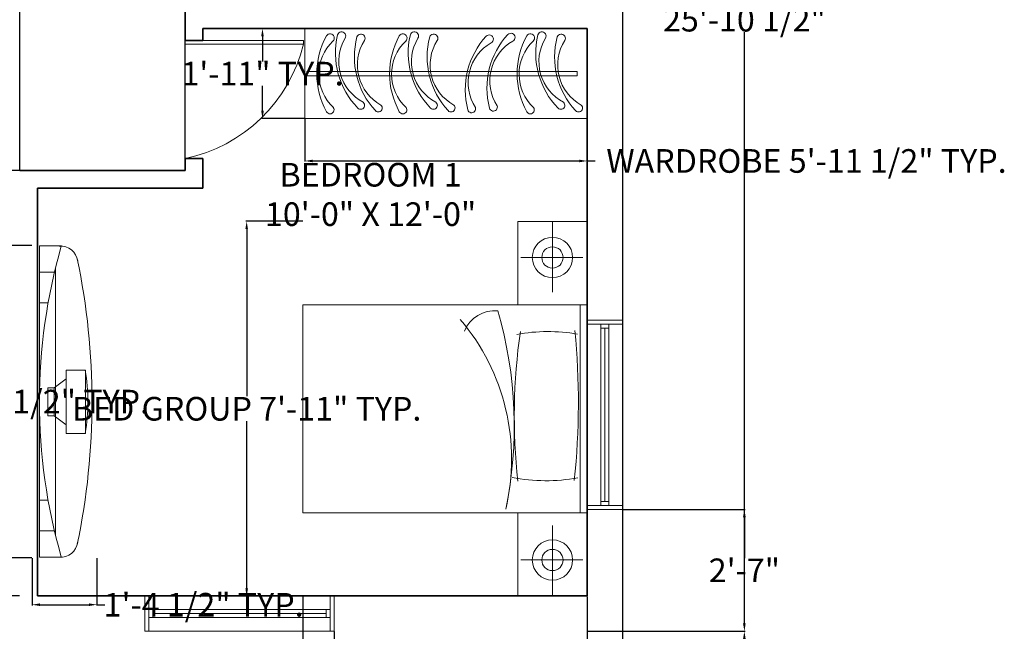
# Model space of a CAD drawing. Units: inches. Extents: x 84 to 590, y 32 to 648.
# Tile 4 of 6: x 340 to 590, y 245 to 401. Entities that reach past the tile are written whole.
import ezdxf

# ---------------------------------------------------------------- set-up
doc = ezdxf.new("R2010")
doc.units = ezdxf.units.IN
doc.header["$MEASUREMENT"] = 0
for name, color, linetype, lineweight in [('A-ANNO-DIMS', 2, 'Continuous', 18), ('A-AREA-IDEN', 7, 'Continuous', 18), ('A-DOOR', 4, 'Continuous', 18), ('A-FLOR-CASE', 9, 'Continuous', 18), ('A-FURN', 8, 'Continuous', 18), ('A-GLAZ', 4, 'Continuous', 18), ('A-WALL', 7, 'Continuous', 35), ('C-PROP', 7, 'Continuous', 30)]:
    doc.layers.add(name, color=color, linetype=linetype, lineweight=lineweight)
doc.styles.get("Standard").update_dxf_attribs({"font": 'arial.ttf'})
doc.dimstyles.get("Standard").update_dxf_attribs({"dimtxt": 6, "dimasz": 2, "dimexe": 0.18, "dimexo": 0.0625, "dimgap": 0.09, "dimtad": 0, "dimtih": 1, "dimtoh": 1, "dimdec": 0, "dimzin": 0, "dimdsep": 46, "dimlunit": 4, "dimtxsty": 'Standard', "dimcen": 0.09, "dimadec": 0, "dimazin": 0, "dimtfac": 1, "dimtdec": 0, "dimtofl": 0, "dimtmove": 0, "dimatfit": 3, "dimfxl": 1, "dimtolj": 1, "dimtzin": 0, "dimarcsym": 1})

# ---------------------------------------------------------------- blocks, each defined once
blk = doc.blocks.new('DOOR')
for p, q in [((185.51, 1128.53), (185.51, 1098.53)), ((185.51, 1128.53), (186.51, 1128.53)), ((186.51, 1098.53), (186.51, 1128.53)), ((186.51, 1098.53), (156.51, 1098.53))]:
    blk.add_line(p, q)
blk.add_arc((194.73, 1090.6), 39.03, 103.6607, 168.2814)
blk = doc.blocks.new('CVBNM')
for p, q in [((388.24, 1592.71), (388.24, 1565.71)), ((420.64, 1592.71), (388.24, 1592.71)), ((420.64, 1592.71), (420.64, 1568.41)), ((420.64, 1482.01), (420.64, 1592.71)), ((501.64, 1592.71), (420.64, 1592.71)), ((420.64, 1565.71), (420.64, 1592.71)), ((501.64, 1592.71), (501.64, 1568.41)), ((501.64, 1592.71), (501.64, 1568.41)), ((501.64, 1482.01), (501.64, 1592.71)), ((501.64, 1565.71), (501.64, 1592.71)), ((501.64, 1592.71), (534.04, 1592.71)), ((534.04, 1592.71), (534.04, 1565.71)), ((402.21, 1579.21), (402.21, 1591.06)), ((501.64, 1590.01), (420.64, 1590.01)), ((520.07, 1579.21), (520.07, 1591.06)), ((402.21, 1579.21), (388.08, 1579.21)), ((402.21, 1579.21), (415.71, 1579.21)), ((402.21, 1579.21), (402.21, 1566.9)), ((520.07, 1579.21), (506.57, 1579.21)), ((520.07, 1579.21), (534.21, 1579.21)), ((520.07, 1579.21), (520.07, 1566.9)), ((388.24, 1565.71), (420.64, 1565.71)), ((534.04, 1565.71), (501.64, 1565.71)), ((501.64, 1482.01), (420.64, 1482.01))]:
    blk.add_line(p, q)
for centre, radius in [((402.21, 1579.21), 7.85), ((520.07, 1579.21), 7.85), ((402.21, 1579.21), 4.15), ((520.07, 1579.21), 4.15)]:
    blk.add_circle(centre, radius)
for centre, radius, start, end in [((458.61, 1300.37), 288.94, 83.953, 95.5626), ((496.51, 1577.48), 65.44, 169.9145, 190.6851), ((419.34, 1576.61), 69.84, 349.1761, 10.2706), ((464.08, 1794.56), 230.23, 261.7649, 276.2896), ((467.83, 1404.8), 159.53, 78.2462, 106.3473), ((480.78, 1479.19), 84.09, 76.5636, 130.3236), ((435.77, 1556.83), 12.88, 175.3269, 247.5588)]:
    blk.add_arc(centre, radius, start, end)
blk = doc.blocks.new('A$C20D7642B')
for p, q in [((0, 1879.7), (0, 0)), ((600, 1879.7), (0, 1879.7)), ((600, 1879.7), (600, 0)), ((285.2, 14), (285.2, 1812.3)), ((285.2, 1812.3), (316, 1812.3)), ((316, 1812.3), (316, 14)), ((340, 0), (0, 0)), ((316, 14), (285.2, 14)), ((340, 0), (600, 0))]:
    blk.add_line(p, q)
for centre, radius, start, end in [((242.6, 1988.3), 305.1, 237.78554, 330.91711), ((529.2, 1822.6), 26.4, 312.06888, 138.87685), ((189.7, 2189.4), 526.2, 255.30638, 312.74923), ((64.5, 1707), 27.8, 56.33784, 252.73759), ((220.7, 1863.8), 305.1, 239.17077, 332.30233), ((511.2, 1705.1), 26.4, 313.4541, 140.26207), ((163, 2063.5), 526.2, 256.69161, 314.13445), ((49.5, 1578.3), 27.8, 57.72306, 254.12281), ((62.8, 1501.9), 27.8, 42.31003, 238.70978), ((303.8, 1731.6), 305.1, 223.75774, 316.8893), ((541.6, 1501.4), 26.4, 298.04107, 124.84904), ((301.2, 1939.5), 526.2, 241.27858, 298.72142), ((59.1, 1372.1), 27.8, 28.28014, 224.67989), ((348.6, 1536.6), 305.1, 209.72784, 302.85941), ((396.5, 1738.9), 526.2, 227.24868, 284.69153), ((70.6, 1227.4), 27.8, 28.28014, 224.67989), ((523.6, 1255.6), 26.4, 284.01118, 110.81915), ((408, 1594.2), 526.2, 227.24868, 284.69153), ((360, 1391.9), 305.1, 209.72784, 302.85941), ((535, 1110.9), 26.4, 284.01118, 110.81915), ((242.6, 1139.3), 305.1, 237.78554, 330.91711), ((529.2, 973.6), 26.4, 312.06888, 138.87685), ((189.7, 1340.3), 526.2, 255.30638, 312.74923), ((64.5, 857.9), 27.8, 56.33784, 252.73759), ((220.7, 1014.8), 305.1, 239.17077, 332.30233), ((511.2, 856), 26.4, 313.4541, 140.26207), ((163, 1214.5), 526.2, 256.69161, 314.13445), ((49.5, 729.2), 27.8, 57.72306, 254.12281), ((62.8, 652.8), 27.8, 42.31003, 238.70978), ((303.8, 882.6), 305.1, 223.75774, 316.8893), ((541.6, 652.4), 26.4, 298.04107, 124.84904), ((301.2, 1090.5), 526.2, 241.27858, 298.72142), ((189.7, 856), 526.2, 255.30638, 312.74923), ((242.6, 655), 305.1, 237.78554, 330.91711), ((529.2, 489.2), 26.4, 312.06888, 138.87685), ((64.5, 373.6), 27.8, 56.33784, 252.73759), ((511.2, 371.7), 26.4, 313.4541, 140.26207), ((163, 730.2), 526.2, 256.69161, 314.13445), ((220.7, 530.5), 305.1, 239.17077, 332.30233), ((49.5, 244.9), 27.8, 57.72306, 254.12281), ((62.8, 168.5), 27.8, 42.31003, 238.70978), ((301.2, 606.1), 526.2, 241.27858, 298.72142), ((303.8, 398.3), 305.1, 223.75774, 316.8893), ((541.6, 168), 26.4, 298.04107, 124.84904)]:
    blk.add_arc(centre, radius, start, end)
blk = doc.blocks.new('A$C78AE5658')
for p, q in [((1515, 306), (1515, 524)), ((1515, 524), (2236, 524)), ((2236, 306), (2236, 524)), ((98, 250), (98, 252)), ((98, 250), (98, 0)), ((1515, 306), (2236, 306)), ((1613, 306), (1716, 168)), ((2137, 306), (2034, 168)), ((3648, 250), (3648, 252)), ((3648, 0), (3648, 250)), ((348, 184), (3398, 184)), ((398, 0), (398, 172)), ((2034, 168), (1716, 168)), ((1716, 168), (1716, 98)), ((2034, 168), (2034, 98)), ((3348, 0), (3348, 172)), ((3648, 0), (98, 0)), ((748, 0), (748, 99)), ((2034, 98), (1716, 98)), ((2998, 0), (2998, 99))]:
    blk.add_line(p, q)
blk.add_lwpolyline([(246, 432, -0.103184), (3500, 432, -0.103184)], format="xyb")
for centre, radius, start, end in [((1875, -1675), 2228, 80.6925, 99.3075), ((298, 239), 200, 98.4687, 183.693), ((3449, 239), 200, 356.307, 81.5313), ((1873, 6426), 6426, 253.9658, 286.0342)]:
    blk.add_arc(centre, radius, start, end)
blk = doc.blocks.new('WIND')
for p, q in [((-51.89, 1021.98), (-99.89, 1021.98)), ((-99.89, 1021.98), (-99.89, 1012.98)), ((-98.89, 1021.98), (-98.89, 1012.98)), ((-52.89, 1012.98), (-52.89, 1021.98)), ((-51.89, 1012.98), (-51.89, 1021.98)), ((-98.89, 1018.48), (-52.89, 1018.48)), ((-97.89, 1018.48), (-97.89, 1016.48)), ((-97.89, 1017.48), (-53.89, 1017.48)), ((-53.89, 1016.48), (-53.89, 1018.48)), ((-98.89, 1016.48), (-52.89, 1016.48)), ((-99.89, 1012.98), (-51.89, 1012.98))]:
    blk.add_line(p, q)
blk = doc.blocks.new('*D23')
at = {"layer": 'A-ANNO-DIMS', "color": 0, "lineweight": -2, "transparency": 16777216}
for p, q in [((411.85, 349.43), (397.45, 349.43)), ((397.63, 347.43), (397.63, 305.03)), ((397.63, 256.23), (397.63, 298.64)), ((411.85, 254.23), (397.45, 254.23))]:
    blk.add_line(p, q, dxfattribs=at)
at = {"layer": 'A-ANNO-DIMS', "color": 0, "transparency": 16777216}
for points in [[(397.3, 347.43), (397.96, 347.43), (397.63, 349.43)], [(397.3, 256.23), (397.96, 256.23), (397.63, 254.23)]]:
    blk.add_solid(points, dxfattribs=at)
at = {"layer": 'Defpoints', "color": 0, "transparency": 16777216}
for p in [(411.91, 349.43), (397.63, 254.23), (411.91, 254.23)]:
    blk.add_point(p, dxfattribs=at)
at = {"layer": 'A-ANNO-DIMS', "color": 0, "transparency": 16777216, "insert": (397.63, 301.83), "char_height": 6, "attachment_point": 5}
blk.add_mtext('\\A1;BED GROUP 7\'-11" TYP.', dxfattribs=at)
blk = doc.blocks.new('*D24')
at = {"layer": 'A-ANNO-DIMS', "color": 0, "lineweight": -2, "transparency": 16777216}
for p, q in [((411.91, 254.17), (411.91, 239.77)), ((484.03, 254.17), (484.03, 239.77)), ((413.91, 239.95), (429.58, 239.95)), ((482.03, 239.95), (466.36, 239.95))]:
    blk.add_line(p, q, dxfattribs=at)
at = {"layer": 'A-ANNO-DIMS', "color": 0, "transparency": 16777216}
for points in [[(413.91, 240.28), (413.91, 239.62), (411.91, 239.95)], [(482.03, 240.28), (482.03, 239.62), (484.03, 239.95)]]:
    blk.add_solid(points, dxfattribs=at)
at = {"layer": 'Defpoints', "color": 0, "transparency": 16777216}
for p in [(411.91, 254.23), (484.03, 254.23), (484.03, 239.95)]:
    blk.add_point(p, dxfattribs=at)
at = {"layer": 'A-ANNO-DIMS', "color": 0, "transparency": 16777216, "insert": (447.97, 239.95), "char_height": 6, "attachment_point": 5}
blk.add_mtext('\\A1;6\'-0" TYP.', dxfattribs=at)
blk = doc.blocks.new('*D25')
at = {"layer": 'A-ANNO-DIMS', "color": 0, "lineweight": -2, "transparency": 16777216}
for p, q in [((343.11, 343.29), (331.1, 343.29)), ((331.28, 341.29), (331.28, 306.83)), ((331.28, 265.98), (331.28, 300.44)), ((343.11, 263.98), (331.1, 263.98))]:
    blk.add_line(p, q, dxfattribs=at)
at = {"layer": 'A-ANNO-DIMS', "color": 0, "transparency": 16777216}
for points in [[(330.95, 341.29), (331.61, 341.29), (331.28, 343.29)], [(330.95, 265.98), (331.61, 265.98), (331.28, 263.98)]]:
    blk.add_solid(points, dxfattribs=at)
at = {"layer": 'Defpoints', "color": 0, "transparency": 16777216}
for p in [(343.17, 343.29), (331.28, 263.98), (343.17, 263.98)]:
    blk.add_point(p, dxfattribs=at)
at = {"layer": 'A-ANNO-DIMS', "color": 0, "transparency": 16777216, "insert": (331.28, 303.64), "char_height": 6, "attachment_point": 5}
blk.add_mtext('\\A1;TV UNIT 6\'-7 1/2" TYP.', dxfattribs=at)
blk = doc.blocks.new('*D26')
at = {"layer": 'A-ANNO-DIMS', "color": 0, "lineweight": -2, "transparency": 16777216}
for p, q in [((343.17, 263.92), (343.17, 251.91)), ((359.62, 263.92), (359.62, 251.91)), ((345.17, 252.09), (357.62, 252.09)), ((359.62, 252.09), (361.62, 252.09))]:
    blk.add_line(p, q, dxfattribs=at)
at = {"layer": 'A-ANNO-DIMS', "color": 0, "transparency": 16777216}
for points in [[(345.17, 252.42), (345.17, 251.76), (343.17, 252.09)], [(357.62, 252.42), (357.62, 251.76), (359.62, 252.09)]]:
    blk.add_solid(points, dxfattribs=at)
at = {"layer": 'Defpoints', "color": 0, "transparency": 16777216}
for p in [(343.17, 263.98), (359.62, 263.98), (359.62, 252.09)]:
    blk.add_point(p, dxfattribs=at)
at = {"layer": 'A-ANNO-DIMS', "color": 0, "transparency": 16777216, "insert": (386.71, 252.09), "char_height": 6, "attachment_point": 5}
blk.add_mtext('\\A1;1\'-4 1/2" TYP.', dxfattribs=at)
blk = doc.blocks.new('*D27')
at = {"layer": 'A-ANNO-DIMS', "color": 0, "lineweight": -2, "transparency": 16777216}
for p, q in [((412.39, 375.41), (412.39, 364.55)), ((484.03, 375.41), (484.03, 364.55)), ((414.39, 364.73), (482.03, 364.73)), ((484.03, 364.73), (486.03, 364.73))]:
    blk.add_line(p, q, dxfattribs=at)
at = {"layer": 'A-ANNO-DIMS', "color": 0, "transparency": 16777216}
for points in [[(414.39, 365.06), (414.39, 364.39), (412.39, 364.73)], [(482.03, 365.06), (482.03, 364.39), (484.03, 364.73)]]:
    blk.add_solid(points, dxfattribs=at)
at = {"layer": 'Defpoints', "color": 0, "transparency": 16777216}
for p in [(412.39, 375.47), (484.03, 375.47), (484.03, 364.73)]:
    blk.add_point(p, dxfattribs=at)
at = {"layer": 'A-ANNO-DIMS', "color": 0, "transparency": 16777216, "insert": (539.69, 364.73), "char_height": 6, "attachment_point": 5}
blk.add_mtext('\\A1;WARDROBE 5\'-11 1/2" TYP.', dxfattribs=at)
blk = doc.blocks.new('*D28')
at = {"layer": 'A-ANNO-DIMS', "color": 0, "lineweight": -2, "transparency": 16777216}
for p, q in [((412.33, 398.34), (401.46, 398.34)), ((401.64, 396.34), (401.64, 390.01)), ((401.64, 377.47), (401.64, 383.8)), ((412.33, 375.47), (401.46, 375.47))]:
    blk.add_line(p, q, dxfattribs=at)
at = {"layer": 'A-ANNO-DIMS', "color": 0, "transparency": 16777216}
for points in [[(401.31, 396.34), (401.98, 396.34), (401.64, 398.34)], [(401.31, 377.47), (401.98, 377.47), (401.64, 375.47)]]:
    blk.add_solid(points, dxfattribs=at)
at = {"layer": 'Defpoints', "color": 0, "transparency": 16777216}
for p in [(412.39, 398.34), (401.64, 375.47), (412.39, 375.47)]:
    blk.add_point(p, dxfattribs=at)
at = {"layer": 'A-ANNO-DIMS', "color": 0, "transparency": 16777216, "insert": (401.64, 386.9), "char_height": 6, "attachment_point": 5}
blk.add_mtext('\\A1;1\'-11" TYP.', dxfattribs=at)
blk = doc.blocks.new('*D44')
at = {"layer": 'A-ANNO-DIMS', "color": 0, "lineweight": -2, "transparency": 16777216}
for p, q in [((484.09, 555.84), (524.11, 555.84)), ((523.93, 553.84), (523.93, 403.78)), ((523.93, 247.34), (523.93, 397.4)), ((484.09, 245.34), (524.11, 245.34))]:
    blk.add_line(p, q, dxfattribs=at)
at = {"layer": 'A-ANNO-DIMS', "color": 0, "transparency": 16777216}
for points in [[(523.59, 553.84), (524.26, 553.84), (523.93, 555.84)], [(523.59, 247.34), (524.26, 247.34), (523.93, 245.34)]]:
    blk.add_solid(points, dxfattribs=at)
at = {"layer": 'Defpoints', "color": 0, "transparency": 16777216}
for p in [(484.03, 555.84), (484.03, 245.34), (523.93, 245.34)]:
    blk.add_point(p, dxfattribs=at)
at = {"layer": 'A-ANNO-DIMS', "color": 0, "transparency": 16777216, "insert": (523.93, 400.59), "char_height": 6, "attachment_point": 5}
blk.add_mtext('\\A1;25\'-10 1/2"', dxfattribs=at)
blk = doc.blocks.new('*D45')
at = {"layer": 'A-ANNO-DIMS', "color": 0, "lineweight": -2, "transparency": 16777216}
for p, q in [((484.09, 245.34), (524.11, 245.34)), ((523.93, 243.34), (523.93, 177.99)), ((523.93, 106.34), (523.93, 171.68)), ((493.09, 104.34), (524.11, 104.34))]:
    blk.add_line(p, q, dxfattribs=at)
at = {"layer": 'A-ANNO-DIMS', "color": 0, "transparency": 16777216}
for points in [[(523.59, 243.34), (524.26, 243.34), (523.93, 245.34)], [(523.59, 106.34), (524.26, 106.34), (523.93, 104.34)]]:
    blk.add_solid(points, dxfattribs=at)
at = {"layer": 'Defpoints', "color": 0, "transparency": 16777216}
for p in [(484.03, 245.34), (493.03, 104.34), (523.93, 104.34)]:
    blk.add_point(p, dxfattribs=at)
at = {"layer": 'A-ANNO-DIMS', "color": 0, "transparency": 16777216, "insert": (523.93, 174.84), "char_height": 6, "attachment_point": 5}
blk.add_mtext('\\A1;11\'-9"', dxfattribs=at)
blk = doc.blocks.new('*D55')
at = {"layer": 'A-ANNO-DIMS', "color": 0, "lineweight": -2, "transparency": 16777216}
for p, q in [((493.09, 276.3), (524.11, 276.3)), ((523.93, 274.3), (523.93, 263.92)), ((523.93, 247.34), (523.93, 257.72)), ((484.09, 245.34), (524.11, 245.34))]:
    blk.add_line(p, q, dxfattribs=at)
at = {"layer": 'A-ANNO-DIMS', "color": 0, "transparency": 16777216}
for points in [[(523.59, 274.3), (524.26, 274.3), (523.93, 276.3)], [(523.59, 247.34), (524.26, 247.34), (523.93, 245.34)]]:
    blk.add_solid(points, dxfattribs=at)
at = {"layer": 'Defpoints', "color": 0, "transparency": 16777216}
for p in [(493.03, 276.3), (523.93, 276.3), (484.03, 245.34)]:
    blk.add_point(p, dxfattribs=at)
at = {"layer": 'A-ANNO-DIMS', "color": 0, "transparency": 16777216, "insert": (523.93, 260.82), "char_height": 6, "attachment_point": 5}
blk.add_mtext('\\A1;2\'-7"', dxfattribs=at)
blk = doc.blocks.new('*D59')
at = {"layer": 'A-ANNO-DIMS', "color": 0, "lineweight": -2, "transparency": 16777216}
for p, q in [((419.82, 245.28), (419.82, 73.26)), ((484.03, 245.28), (484.03, 73.26)), ((421.82, 73.44), (443.86, 73.44)), ((482.03, 73.44), (459.99, 73.44))]:
    blk.add_line(p, q, dxfattribs=at)
at = {"layer": 'A-ANNO-DIMS', "color": 0, "transparency": 16777216}
for points in [[(421.82, 73.77), (421.82, 73.1), (419.82, 73.44)], [(482.03, 73.77), (482.03, 73.1), (484.03, 73.44)]]:
    blk.add_solid(points, dxfattribs=at)
at = {"layer": 'Defpoints', "color": 0, "transparency": 16777216}
for p in [(419.82, 245.34), (484.03, 245.34), (484.03, 73.44)]:
    blk.add_point(p, dxfattribs=at)
at = {"layer": 'A-ANNO-DIMS', "color": 0, "transparency": 16777216, "insert": (451.92, 73.44), "char_height": 6, "attachment_point": 5}
blk.add_mtext('\\A1;5\'-4"', dxfattribs=at)
blk = doc.blocks.new('*D60')
at = {"layer": 'A-ANNO-DIMS', "color": 0, "lineweight": -2, "transparency": 16777216}
for p, q in [((340.03, 362.4), (340.03, 639.42)), ((342.03, 639.24), (352.97, 639.24)), ((380.03, 639.24), (369.09, 639.24)), ((382.03, 362.4), (382.03, 639.42))]:
    blk.add_line(p, q, dxfattribs=at)
at = {"layer": 'A-ANNO-DIMS', "color": 0, "transparency": 16777216}
for points in [[(342.03, 639.57), (342.03, 638.9), (340.03, 639.24)], [(380.03, 639.57), (380.03, 638.9), (382.03, 639.24)]]:
    blk.add_solid(points, dxfattribs=at)
at = {"layer": 'Defpoints', "color": 0, "transparency": 16777216}
for p in [(382.03, 639.24), (340.03, 362.34), (382.03, 362.34)]:
    blk.add_point(p, dxfattribs=at)
at = {"layer": 'A-ANNO-DIMS', "color": 0, "transparency": 16777216, "insert": (361.03, 639.24), "char_height": 6, "attachment_point": 5}
blk.add_mtext('\\A1;3\'-6"', dxfattribs=at)
blk = doc.blocks.new('*D61')
at = {"layer": 'A-ANNO-DIMS', "color": 0, "lineweight": -2, "transparency": 16777216}
for p, q in [((339.97, 362.34), (101.95, 362.34)), ((102.13, 360.34), (102.13, 311.49)), ((102.13, 256.34), (102.13, 305.18)), ((339.97, 254.34), (101.95, 254.34))]:
    blk.add_line(p, q, dxfattribs=at)
at = {"layer": 'A-ANNO-DIMS', "color": 0, "transparency": 16777216}
for points in [[(101.79, 360.34), (102.46, 360.34), (102.13, 362.34)], [(101.79, 256.34), (102.46, 256.34), (102.13, 254.34)]]:
    blk.add_solid(points, dxfattribs=at)
at = {"layer": 'Defpoints', "color": 0, "transparency": 16777216}
for p in [(102.13, 362.34), (340.03, 362.34), (340.03, 254.34)]:
    blk.add_point(p, dxfattribs=at)
at = {"layer": 'A-ANNO-DIMS', "color": 0, "transparency": 16777216, "insert": (102.13, 308.34), "char_height": 6, "attachment_point": 5}
blk.add_mtext('\\A1;9\'-0"', dxfattribs=at)

msp = doc.modelspace()

# ---------------------------------------------------------------- linework, layer by layer
at = {"layer": 'A-WALL'}
for p, q in [((382.03, 398.34), (382.03, 408.84)), ((382.03, 398.34), (382.03, 395.34)), ((386.53, 398.34), (484.03, 398.34)), ((386.53, 398.34), (386.53, 395.34)), ((484.03, 398.34), (484.03, 254.34)), ((382.03, 395.34), (386.53, 395.34)), ((382.03, 365.34), (386.53, 365.34)), ((382.03, 365.34), (382.03, 362.34)), ((386.53, 365.34), (386.53, 357.84)), ((382.03, 362.34), (340.03, 362.34)), ((344.53, 254.34), (344.53, 357.84)), ((386.53, 357.84), (344.53, 357.84)), ((344.53, 254.34), (484.03, 254.34))]:
    msp.add_line(p, q, dxfattribs=at)
at = {"layer": 'C-PROP'}
msp.add_line((493.03, 608.34), (493.03, 104.34), dxfattribs=at)

# ---------------------------------------------------------------- block references
at = {"layer": 'A-DOOR', "xscale": -1, "rotation": 270}
msp.add_blockref('DOOR', (-716.5, 208.83), dxfattribs=at)
at = {"layer": 'A-FLOR-CASE', "xscale": 0.0381118678123285, "yscale": 0.0381118678123285, "zscale": 0.0381118678123285, "rotation": 270}
msp.add_blockref('A$C20D7642B', (412.39, 398.34), dxfattribs=at)
at = {"layer": 'A-FURN', "rotation": 270}
for name, p, xscale, yscale, zscale in [('CVBNM', (-553.6, 602.26), 0.6514848881435277, 0.6514848881435277, 0.6514848881435277), ('A$C78AE5658', (345.03, 345.33), 0.0222542726180731, 0.0222542726180731, 0.0222542726180731)]:
    msp.add_blockref(name, p, dxfattribs=dict(at, xscale=xscale, yscale=yscale, zscale=zscale))
at = {"layer": 'A-GLAZ', "rotation": 270}
msp.add_blockref('WIND', (-528.95, 224.4), dxfattribs=at)
at = {"layer": 'A-GLAZ'}
msp.add_blockref('WIND', (471.71, -767.64), dxfattribs=at)

# ---------------------------------------------------------------- texts
at = {"layer": 'A-AREA-IDEN', "insert": (387.96, 364.23), "char_height": 6, "attachment_point": 1}
msp.add_mtext_dynamic_manual_height_columns('\\pxqc;BEDROOM 1\\P10\'-0" X 12\'-0"', width=82.2238, gutter_width=30, heights=[0], dxfattribs=at)

# ---------------------------------------------------------------- dimensions: what is measured, and where the dimension line sits
at = {"layer": 'A-ANNO-DIMS'}
for base, p1, p2, picture, middle in [((382.03, 639.24), (340.03, 362.34), (382.03, 362.34), '*D60', (361.03, 639.24)), ((484.03, 73.44), (419.82, 245.34), (484.03, 245.34), '*D59', (451.92, 73.44))]:
    dim = msp.add_linear_dim(base=base, p1=p1, p2=p2, dimstyle='Standard', override={"dimdec": 1, "dimlfac": 1, "dimrnd": 0, "dimzin": 1, "dimdsep": 46, "dimlunit": 4, "dimfrac": 2}, dxfattribs=at)
    dim.commit()
    dim.dimension.update_dxf_attribs({"geometry": picture, "text_midpoint": middle})
for base, p1, p2, picture, middle in [((523.93, 245.34), (484.03, 555.84), (484.03, 245.34), '*D44', (523.93, 400.59)), ((102.13, 362.34), (340.03, 254.34), (340.03, 362.34), '*D61', (102.13, 308.34)), ((523.93, 276.3), (484.03, 245.34), (493.03, 276.3), '*D55', (523.93, 260.82)), ((523.93, 104.34), (484.03, 245.34), (493.03, 104.34), '*D45', (523.93, 174.84))]:
    dim = msp.add_linear_dim(base=base, p1=p1, p2=p2, angle=90, dimstyle='Standard', override={"dimdec": 1, "dimlfac": 1, "dimrnd": 0, "dimzin": 1, "dimdsep": 46, "dimlunit": 4, "dimfrac": 2}, dxfattribs=at)
    dim.commit()
    dim.dimension.update_dxf_attribs({"geometry": picture, "text_midpoint": middle})
for base, p1, p2, text, picture, middle in [((401.64, 375.47), (412.39, 398.34), (412.39, 375.47), '<> TYP.', '*D28', (401.64, 386.9)), ((397.63, 254.23), (411.91, 349.43), (411.91, 254.23), 'BED GROUP <> TYP.', '*D23', (397.63, 301.83)), ((331.28, 263.98), (343.17, 343.29), (343.17, 263.98), 'TV UNIT <> TYP.', '*D25', (331.28, 303.64))]:
    dim = msp.add_linear_dim(base=base, p1=p1, p2=p2, angle=270, text=text, dimstyle='Standard', override={"dimdec": 1, "dimlfac": 1, "dimrnd": 0, "dimzin": 1, "dimdsep": 46, "dimlunit": 4, "dimfrac": 2}, dxfattribs=at)
    dim.commit()
    dim.dimension.update_dxf_attribs({"geometry": picture, "text_midpoint": middle})
for base, p1, p2, text, picture, middle in [((484.03, 364.73), (412.39, 375.47), (484.03, 375.47), 'WARDROBE <> TYP.', '*D27', (539.69, 364.73)), ((359.6238, 252.0897), (343.1746, 263.9848), (359.6238, 263.9848), '<> TYP.', '*D26', (386.7084, 252.0897)), ((484.03, 239.95), (411.91, 254.23), (484.03, 254.23), '<> TYP.', '*D24', (447.97, 239.95))]:
    dim = msp.add_linear_dim(base=base, p1=p1, p2=p2, text=text, dimstyle='Standard', override={"dimdec": 1, "dimlfac": 1, "dimrnd": 0, "dimzin": 1, "dimdsep": 46, "dimlunit": 4, "dimfrac": 2}, dxfattribs=at)
    dim.commit()
    dim.dimension.update_dxf_attribs({"geometry": picture, "text_midpoint": middle})

doc.saveas('drawing.dxf')
